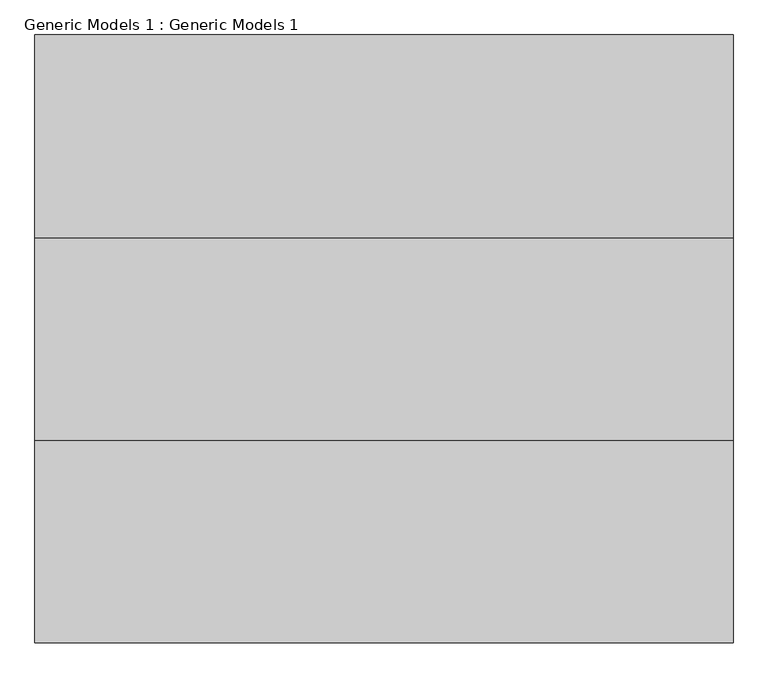
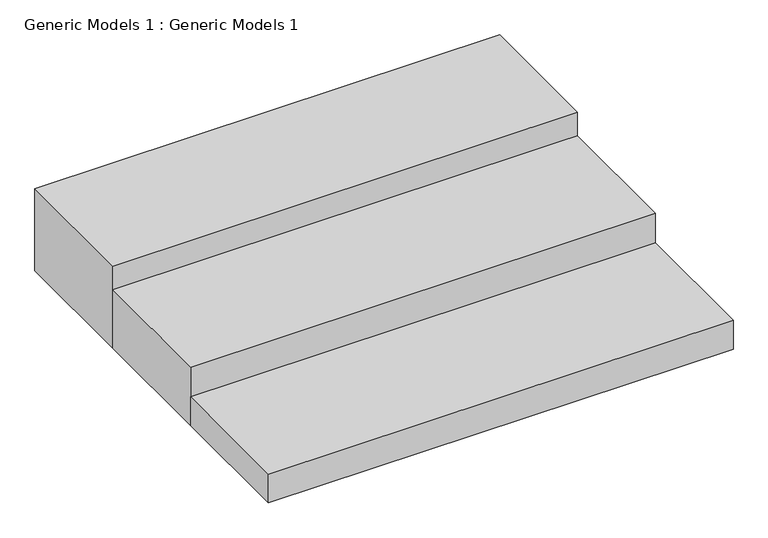
"""IFC4 building model written with IfcOpenShell, lengths in millimetres: proxy geometry, Generic Models 1 : Generic Models 1."""

from ifc_helpers import new_model, si_unit, frame, origin, place, context, project, spatial, polyline, outline, extrude, source, transform, mapped, element, save


def generic_models_1_generic_models_1_13bb2270(model_context):
    return source(origin(), model_context, "Body", "SweptSolid", [
        extrude(outline(polyline([(4413.25, 909.2371517), (5581.65, 909.2371517), (5581.65, 570.1057276), (4413.25, 570.1057276), (4413.25, 909.2371517)])), frame((0.0, 0.0, -76.2), z_axis=(0.0, 0.0, 1.0), x_axis=(1.0, 0.0, 0.0)), (0.0, 0.0, 1.0), 76.2),
        extrude(outline(polyline([(4413.25, 1248.3685759), (5581.65, 1248.3685759), (5581.65, 909.2371517), (4413.25, 909.2371517), (4413.25, 1248.3685759)])), frame((0.0, 0.0, -76.2), z_axis=(0.0, 0.0, 1.0), x_axis=(1.0, 0.0, 0.0)), (0.0, 0.0, 1.0), 155.4569998),
        extrude(outline(polyline([(4413.25, 1587.5), (5581.65, 1587.5), (5581.65, 1248.3685759), (4413.25, 1248.3685759), (4413.25, 1587.5)])), frame((0.0, 0.0, -76.2), z_axis=(0.0, 0.0, 1.0), x_axis=(1.0, 0.0, 0.0)), (0.0, 0.0, 1.0), 218.1410515),
    ])


if __name__ == "__main__":
    model = new_model("IFC4")
    model_context = context("Model", 3, world=origin())
    ifc_project = project(units=[si_unit("LENGTHUNIT", "METRE", prefix="MILLI")], contexts=[model_context])
    site = spatial("IfcSite", under=ifc_project)
    building = spatial("IfcBuilding", under=site)
    placement = place(None, origin())
    generic_models_1_generic_models_1_shape = generic_models_1_generic_models_1_13bb2270(model_context)
    element("IfcBuildingElementProxy", 1, Name="Generic Models 1 : Generic Models 1", ObjectType="Generic Models 1 : Generic Models 1", at=placement, inside=building, context=model_context, shape_type="MappedRepresentation", body=[
        mapped(generic_models_1_generic_models_1_shape, transform((0.0, 0.0, 0.0), x_axis=(1.0, 0.0, 0.0), y_axis=(0.0, 1.0, 0.0), z_axis=(0.0, 0.0, 1.0))),
    ])
    save(model, "model.ifc")

# Revit data of these elements
# Element 1 (IfcBuildingElementProxy, "Generic Models 1 : Generic Models 1")
#   Materials on its faces: "Cherry"
# Materials
#   "Cherry": class "Wood", colour RGB 226 177 128, transparency 0, Description = "Prunus Serotina", Cost = 0
